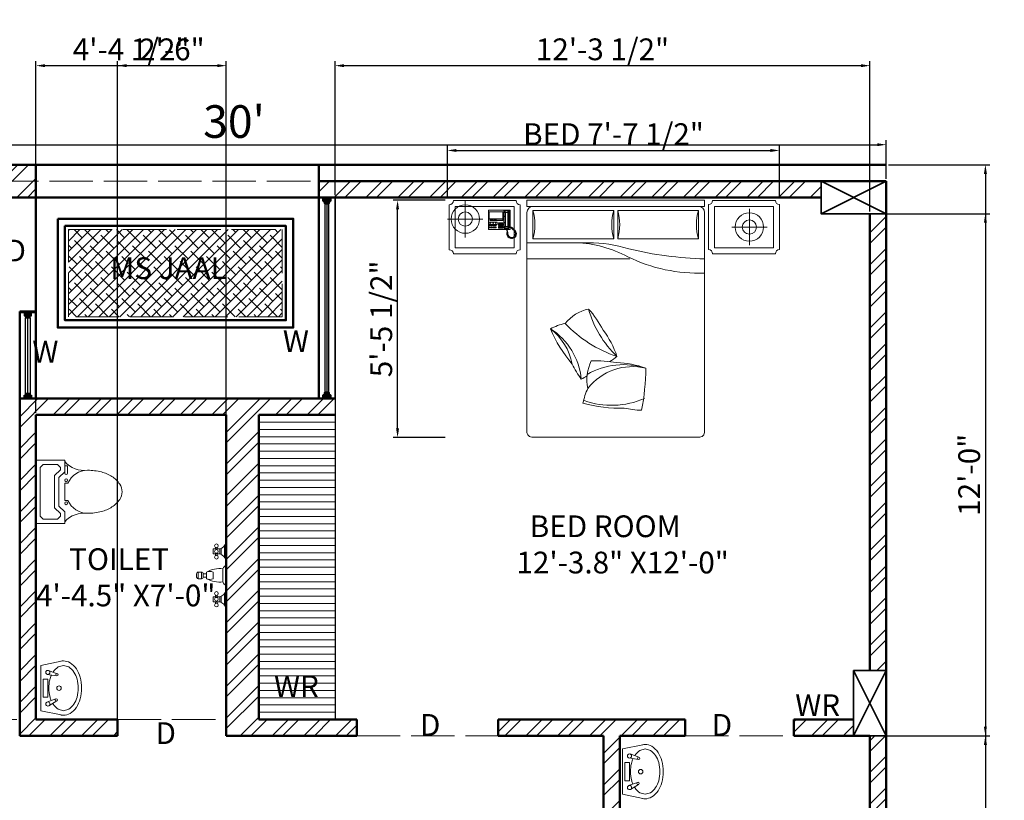
# Model space of a CAD drawing. Units: millimetres. Extents: x 4237 to 5109, y 21391 to 22486.
# Tile 17 of 17: x 4833 to 5105, y 22265 to 22481. Entities that reach past the tile are written whole.
import ezdxf

# ---------------------------------------------------------------- set-up
doc = ezdxf.new("R2010")
doc.units = ezdxf.units.MM
doc.linetypes.add('ACAD_ISO02W100', pattern=[15, 12, -3])
for name, color, linetype, lineweight in [('A-ANNO-DIMS', 2, 'Continuous', 18), ('A-ANNO-TEXT', 7, 'Continuous', 18), ('A-AREA-IDEN', 3, 'Continuous', 18), ('A-FLOR-OVHD', 1, 'ACAD_ISO02W100', 18), ('A-FURN', 8, 'Continuous', 18), ('A-FURN-CASE', 31, 'Continuous', 13), ('A-WALL', 7, 'Continuous', 50), ('A-WALL-PATT', 252, 'Continuous', 13), ('column', 102, 'Continuous', 35), ('windows', 140, 'Continuous', 25)]:
    doc.layers.add(name, color=color, linetype=linetype, lineweight=lineweight)
doc.styles.get("Standard").update_dxf_attribs({"font": 'arial.ttf'})
doc.dimstyles.new('ISO-25', dxfattribs={"dimtxt": 6, "dimasz": 2.5, "dimexe": 1.25, "dimexo": 0.625, "dimtad": 1, "dimdec": 1, "dimlunit": 4, "dimtxsty": 'Standard', "dimcen": 2.5, "dimadec": 0, "dimazin": 0, "dimtfac": 1, "dimtdec": 1, "dimtmove": 0, "dimatfit": 3, "dimfxl": 1, "dimarcsym": 0})

# ---------------------------------------------------------------- blocks, each defined once
blk = doc.blocks.new('A$C07097A50')
for p, q in [((0.0503, 1.9981), (0.5803, 1.9981)), ((0.1513, 1.6872), (0.1513, 1.9968)), ((0.6716, 1.9489), (0.6716, 2.0001)), ((0.6716, 2.0001), (2.1719, 2.0001)), ((2.1719, 1.9489), (2.1719, 2.0001)), ((2.7701, 1.9993), (2.2401, 1.9993)), ((0.0153, 1.9631), (0.0153, 1.5831)), ((0.0653, 1.9481), (0.0653, 1.5981)), ((0.0653, 1.9481), (0.5653, 1.9481)), ((0.3481, 1.9163), (0.3458, 1.914)), ((0.3458, 1.914), (0.3458, 1.7563)), ((0.3481, 1.9163), (0.5287, 1.9163)), ((0.4772, 1.9071), (0.4818, 1.9129)), ((0.4818, 1.9129), (0.5161, 1.9129)), ((0.5161, 1.9129), (0.5218, 1.9071)), ((0.5287, 1.9163), (0.5309, 1.914)), ((0.5309, 1.914), (0.5309, 1.7563)), ((0.5653, 1.9481), (0.5653, 1.5981)), ((0.6153, 1.9631), (0.6153, 1.5831)), ((2.1719, 1.9489), (0.6716, 1.9489)), ((2.2051, 1.9643), (2.2051, 1.5843)), ((2.2551, 1.9493), (2.2551, 1.5993)), ((2.7551, 1.9493), (2.2551, 1.9493)), ((2.5505, 1.6201), (2.5505, 1.9296)), ((2.7551, 1.9493), (2.7551, 1.5993)), ((2.8051, 1.9643), (2.8051, 1.5843)), ((0, 1.8416), (0.3001, 1.8416)), ((0.3526, 1.9037), (0.3526, 1.8431)), ((0.4669, 1.9037), (0.3526, 1.9037)), ((0.3526, 1.8431), (0.4669, 1.8431)), ((0.3572, 1.8409), (0.3572, 1.8294)), ((0.4669, 1.8409), (0.3572, 1.8409)), ((0.3572, 1.8294), (0.4669, 1.8294)), ((0.3664, 1.8409), (0.3664, 1.8294)), ((0.3755, 1.8409), (0.3755, 1.8294)), ((0.3846, 1.8409), (0.3846, 1.8294)), ((0.3938, 1.8409), (0.3938, 1.8294)), ((0.4029, 1.8409), (0.4029, 1.8294)), ((0.4121, 1.8409), (0.4121, 1.8294)), ((0.4669, 1.8431), (0.4669, 1.9037)), ((0.4669, 1.8294), (0.4669, 1.8409)), ((0.4772, 1.7688), (0.4772, 1.9071)), ((0.4818, 1.9094), (0.4807, 1.9049)), ((0.4807, 1.9049), (0.4807, 1.874)), ((0.4807, 1.9049), (0.4909, 1.8946)), ((0.4807, 1.874), (0.4829, 1.8683)), ((0.4864, 1.9117), (0.4818, 1.9094)), ((0.4829, 1.8683), (0.4864, 1.8626)), ((0.4921, 1.8969), (0.4864, 1.9117)), ((0.4864, 1.9117), (0.5138, 1.9117)), ((0.4864, 1.8626), (0.4875, 1.8546)), ((0.4875, 1.8546), (0.4875, 1.8431)), ((0.4875, 1.8214), (0.4875, 1.8431)), ((0.4909, 1.8946), (0.4921, 1.8969)), ((0.4909, 1.8431), (0.4909, 1.8946)), ((0.4909, 1.8431), (0.4909, 1.7814)), ((0.5081, 1.8969), (0.4921, 1.8969)), ((0.5081, 1.8969), (0.5138, 1.9117)), ((0.5092, 1.8946), (0.5081, 1.8969)), ((0.5195, 1.9049), (0.5092, 1.8946)), ((0.5092, 1.8431), (0.5092, 1.8946)), ((0.5092, 1.8431), (0.5092, 1.7814)), ((0.5138, 1.8626), (0.5127, 1.8546)), ((0.5127, 1.8546), (0.5127, 1.8431)), ((0.5127, 1.8214), (0.5127, 1.8431)), ((0.5138, 1.9117), (0.5184, 1.9094)), ((0.5172, 1.8683), (0.5138, 1.8626)), ((0.5195, 1.874), (0.5172, 1.8683)), ((0.5184, 1.9094), (0.5195, 1.9049)), ((0.5195, 1.9049), (0.5195, 1.874)), ((0.5218, 1.9071), (0.5218, 1.77)), ((0.6716, 1.8977), (0.6716, 0.0512)), ((2.1719, 0.0512), (2.1719, 1.8977)), ((0.3458, 1.7563), (0.3481, 1.754)), ((0.5, 1.754), (0.3481, 1.754)), ((0.4201, 1.8168), (0.3526, 1.8168)), ((0.3526, 1.8168), (0.3526, 1.7963)), ((0.3526, 1.7963), (0.4201, 1.7963)), ((0.3652, 1.7906), (0.3538, 1.7906)), ((0.3538, 1.7906), (0.3538, 1.786)), ((0.3538, 1.786), (0.3652, 1.786)), ((0.3538, 1.7666), (0.3538, 1.7734)), ((0.3538, 1.7734), (0.3652, 1.7734)), ((0.3652, 1.7666), (0.3538, 1.7666)), ((0.3675, 1.8146), (0.3641, 1.8146)), ((0.3641, 1.8146), (0.3641, 1.8111)), ((0.3641, 1.8111), (0.3675, 1.8111)), ((0.3641, 1.802), (0.3641, 1.7986)), ((0.3675, 1.802), (0.3641, 1.802)), ((0.3641, 1.7986), (0.3675, 1.7986)), ((0.3652, 1.786), (0.3652, 1.7906)), ((0.3652, 1.7734), (0.3652, 1.7666)), ((0.3675, 1.8111), (0.3675, 1.8146)), ((0.3675, 1.7986), (0.3675, 1.802)), ((0.3812, 1.7906), (0.3698, 1.7906)), ((0.3698, 1.7906), (0.3698, 1.786)), ((0.3698, 1.786), (0.3812, 1.786)), ((0.3698, 1.7666), (0.3698, 1.7734)), ((0.3698, 1.7734), (0.3812, 1.7734)), ((0.3812, 1.7666), (0.3698, 1.7666)), ((0.3812, 1.786), (0.3812, 1.7906)), ((0.3812, 1.7734), (0.3812, 1.7666)), ((0.3846, 1.8146), (0.3846, 1.8111)), ((0.3881, 1.8146), (0.3846, 1.8146)), ((0.3846, 1.8111), (0.3881, 1.8111)), ((0.3846, 1.802), (0.3846, 1.7986)), ((0.3881, 1.802), (0.3846, 1.802)), ((0.3846, 1.7986), (0.3881, 1.7986)), ((0.3972, 1.7906), (0.3858, 1.7906)), ((0.3858, 1.7906), (0.3858, 1.786)), ((0.3858, 1.786), (0.3972, 1.786)), ((0.3858, 1.7666), (0.3858, 1.7734)), ((0.3858, 1.7734), (0.3972, 1.7734)), ((0.3972, 1.7666), (0.3858, 1.7666)), ((0.3881, 1.8111), (0.3881, 1.8146)), ((0.3881, 1.7986), (0.3881, 1.802)), ((0.3972, 1.786), (0.3972, 1.7906)), ((0.3972, 1.7734), (0.3972, 1.7666)), ((0.4018, 1.7906), (0.4018, 1.786)), ((0.4132, 1.7906), (0.4018, 1.7906)), ((0.4018, 1.786), (0.4132, 1.786)), ((0.4018, 1.7734), (0.4132, 1.7734)), ((0.4018, 1.7666), (0.4018, 1.7734)), ((0.4132, 1.7666), (0.4018, 1.7666)), ((0.4052, 1.8146), (0.4052, 1.8111)), ((0.4086, 1.8146), (0.4052, 1.8146)), ((0.4052, 1.8111), (0.4086, 1.8111)), ((0.4052, 1.802), (0.4052, 1.7986)), ((0.4086, 1.802), (0.4052, 1.802)), ((0.4052, 1.7986), (0.4086, 1.7986)), ((0.4086, 1.8111), (0.4086, 1.8146)), ((0.4086, 1.7986), (0.4086, 1.802)), ((0.4132, 1.786), (0.4132, 1.7906)), ((0.4132, 1.7734), (0.4132, 1.7666)), ((0.4201, 1.7963), (0.4201, 1.8168)), ((0.4304, 1.8111), (0.4395, 1.8111)), ((0.4304, 1.8043), (0.4304, 1.8111)), ((0.4395, 1.8043), (0.4304, 1.8043)), ((0.4304, 1.7986), (0.4395, 1.7986)), ((0.4304, 1.7917), (0.4304, 1.7986)), ((0.4395, 1.7917), (0.4304, 1.7917)), ((0.4304, 1.778), (0.4304, 1.7848)), ((0.4304, 1.7848), (0.4395, 1.7848)), ((0.4395, 1.778), (0.4304, 1.778)), ((0.4304, 1.7723), (0.4395, 1.7723)), ((0.4304, 1.7654), (0.4304, 1.7723)), ((0.4395, 1.7654), (0.4304, 1.7654)), ((0.4395, 1.8111), (0.4395, 1.8043)), ((0.4395, 1.7986), (0.4395, 1.7917)), ((0.4395, 1.7848), (0.4395, 1.778)), ((0.4395, 1.7723), (0.4395, 1.7654)), ((0.4441, 1.8043), (0.4441, 1.8111)), ((0.4441, 1.8111), (0.4532, 1.8111)), ((0.4532, 1.8043), (0.4441, 1.8043)), ((0.4441, 1.7986), (0.4532, 1.7986)), ((0.4441, 1.7917), (0.4441, 1.7986)), ((0.4532, 1.7917), (0.4441, 1.7917)), ((0.4441, 1.778), (0.4441, 1.7848)), ((0.4441, 1.7848), (0.4532, 1.7848)), ((0.4532, 1.778), (0.4441, 1.778)), ((0.4441, 1.7723), (0.4532, 1.7723)), ((0.4441, 1.7654), (0.4441, 1.7723)), ((0.4532, 1.7654), (0.4441, 1.7654)), ((0.4532, 1.8111), (0.4532, 1.8043)), ((0.4532, 1.7986), (0.4532, 1.7917)), ((0.4532, 1.7848), (0.4532, 1.778)), ((0.4532, 1.7723), (0.4532, 1.7654)), ((0.4578, 1.8111), (0.4669, 1.8111)), ((0.4578, 1.8043), (0.4578, 1.8111)), ((0.4669, 1.8043), (0.4578, 1.8043)), ((0.4578, 1.7986), (0.4669, 1.7986)), ((0.4578, 1.7917), (0.4578, 1.7986)), ((0.4669, 1.7917), (0.4578, 1.7917)), ((0.4578, 1.7791), (0.4578, 1.786)), ((0.4578, 1.786), (0.4669, 1.786)), ((0.4669, 1.7791), (0.4578, 1.7791)), ((0.4578, 1.7654), (0.4578, 1.7723)), ((0.4578, 1.7723), (0.4669, 1.7723)), ((0.4669, 1.7654), (0.4578, 1.7654)), ((0.4669, 1.8111), (0.4669, 1.8043)), ((0.4669, 1.7986), (0.4669, 1.7917)), ((0.4669, 1.786), (0.4669, 1.7791)), ((0.4669, 1.7723), (0.4669, 1.7654)), ((0.4829, 1.7631), (0.4772, 1.7688)), ((0.4807, 1.802), (0.4829, 1.8077)), ((0.4807, 1.7711), (0.4807, 1.802)), ((0.4807, 1.7711), (0.4909, 1.7814)), ((0.4818, 1.7666), (0.4807, 1.7711)), ((0.4864, 1.7643), (0.4818, 1.7666)), ((0.4829, 1.8077), (0.4864, 1.8134)), ((0.499, 1.7631), (0.4829, 1.7631)), ((0.4864, 1.8134), (0.4875, 1.8214)), ((0.4921, 1.7791), (0.4864, 1.7643)), ((0.4864, 1.7643), (0.499, 1.7643)), ((0.4909, 1.7814), (0.4921, 1.7791)), ((0.5081, 1.7791), (0.4921, 1.7791)), ((0.5024, 1.7677), (0.4989, 1.7677)), ((0.4989, 1.7677), (0.4991, 1.7578)), ((0.4991, 1.7578), (0.5019, 1.7463)), ((0.5019, 1.7463), (0.5047, 1.7354)), ((0.503, 1.7585), (0.5024, 1.7677)), ((0.5026, 1.7643), (0.5138, 1.7643)), ((0.5161, 1.7631), (0.5027, 1.7631)), ((0.5047, 1.7511), (0.503, 1.7585)), ((0.5287, 1.754), (0.504, 1.754)), ((0.5074, 1.7403), (0.5047, 1.7511)), ((0.5092, 1.7814), (0.5081, 1.7791)), ((0.5081, 1.7791), (0.5138, 1.7643)), ((0.5195, 1.7711), (0.5092, 1.7814)), ((0.5138, 1.8134), (0.5127, 1.8214)), ((0.5172, 1.8077), (0.5138, 1.8134)), ((0.5138, 1.7643), (0.5184, 1.7666)), ((0.5218, 1.77), (0.5161, 1.7631)), ((0.5195, 1.802), (0.5172, 1.8077)), ((0.5184, 1.7666), (0.5195, 1.7711)), ((0.5195, 1.7711), (0.5195, 1.802)), ((0.5309, 1.7563), (0.5287, 1.754)), ((0.5378, 1.7743), (0.5309, 1.7768)), ((0.5309, 1.7723), (0.536, 1.7709)), ((0.536, 1.7709), (0.5406, 1.7672)), ((0.541, 1.7711), (0.5378, 1.7743)), ((0.5406, 1.7672), (0.5418, 1.7656)), ((0.5434, 1.7689), (0.541, 1.7711)), ((0.5442, 1.7658), (0.5418, 1.7634)), ((0.5418, 1.7656), (0.5442, 1.7658)), ((0.5418, 1.7634), (0.5511, 1.7552)), ((0.5477, 1.7705), (0.5434, 1.7689)), ((0.5497, 1.7685), (0.5477, 1.7705)), ((0.5481, 1.765), (0.5497, 1.7685)), ((0.5509, 1.7672), (0.5481, 1.765)), ((0.5539, 1.764), (0.5509, 1.7672)), ((0.5511, 1.7552), (0.5662, 1.7423)), ((0.5515, 1.7574), (0.5539, 1.764)), ((0.5577, 1.7606), (0.5515, 1.7574)), ((0.563, 1.7556), (0.5577, 1.7606)), ((0.5618, 1.7483), (0.563, 1.7556)), ((0.567, 1.7515), (0.5618, 1.7483)), ((0.5714, 1.7469), (0.567, 1.7515)), ((0.5696, 1.7419), (0.5714, 1.7469)), ((2.7018, 1.7745), (2.4017, 1.7745)), ((0.5026, 1.7254), (0.5021, 1.7199)), ((0.5021, 1.7199), (0.5088, 1.7187)), ((0.5088, 1.7187), (0.5023, 1.7148)), ((0.5023, 1.7148), (0.5028, 1.7085)), ((0.5051, 1.728), (0.5026, 1.7254)), ((0.5028, 1.7085), (0.5102, 1.7078)), ((0.5102, 1.7078), (0.5037, 1.7028)), ((0.5037, 1.7028), (0.5067, 1.6974)), ((0.5047, 1.7354), (0.5044, 1.7294)), ((0.5044, 1.7294), (0.5051, 1.728)), ((0.5067, 1.6974), (0.5137, 1.6988)), ((0.5081, 1.7347), (0.5074, 1.7403)), ((0.5079, 1.7287), (0.5081, 1.7347)), ((0.5121, 1.7257), (0.5079, 1.7287)), ((0.5137, 1.6988), (0.5104, 1.6923)), ((0.5104, 1.6923), (0.5139, 1.6882)), ((0.5111, 1.7203), (0.5121, 1.7257)), ((0.5123, 1.7058), (0.5111, 1.7203)), ((0.5211, 1.6947), (0.5123, 1.7058)), ((0.5139, 1.6882), (0.5192, 1.6921)), ((0.5192, 1.6921), (0.5183, 1.6859)), ((0.5183, 1.6859), (0.5227, 1.6831)), ((0.5333, 1.6882), (0.5211, 1.6947)), ((0.5227, 1.6831), (0.5282, 1.6877)), ((0.5282, 1.6877), (0.5276, 1.6801)), ((0.5276, 1.6801), (0.5324, 1.6787)), ((0.5324, 1.6787), (0.5354, 1.6849)), ((0.5472, 1.687), (0.5333, 1.6882)), ((0.5354, 1.6849), (0.5382, 1.6787)), ((0.5382, 1.6787), (0.5421, 1.6782)), ((0.5421, 1.6782), (0.5437, 1.6849)), ((0.5437, 1.6849), (0.5463, 1.6775)), ((0.5463, 1.6775), (0.5507, 1.6787)), ((0.5606, 1.6928), (0.5472, 1.687)), ((0.5507, 1.6787), (0.5509, 1.6849)), ((0.5509, 1.6849), (0.5562, 1.6803)), ((0.5562, 1.6803), (0.5599, 1.6822)), ((0.5592, 1.6891), (0.5641, 1.6831)), ((0.5599, 1.6822), (0.5592, 1.6891)), ((0.5708, 1.7028), (0.5606, 1.6928)), ((0.5641, 1.6831), (0.5678, 1.6863)), ((0.565, 1.6926), (0.5715, 1.6898)), ((0.5678, 1.6863), (0.565, 1.6926)), ((0.5664, 1.7419), (0.574, 1.7201)), ((0.5766, 1.7426), (0.5697, 1.7419)), ((0.574, 1.7201), (0.5708, 1.7028)), ((0.5745, 1.6926), (0.5713, 1.6988)), ((0.5713, 1.6988), (0.578, 1.6967)), ((0.5715, 1.6898), (0.5745, 1.6926)), ((0.572, 1.7331), (0.5787, 1.7356)), ((0.5794, 1.7333), (0.572, 1.7331)), ((0.5743, 1.7076), (0.5814, 1.7074)), ((0.5798, 1.7014), (0.5743, 1.7076)), ((0.5761, 1.7234), (0.581, 1.728)), ((0.5824, 1.7234), (0.5761, 1.7234)), ((0.5764, 1.7155), (0.5835, 1.7176)), ((0.5824, 1.712), (0.5764, 1.7155)), ((0.5787, 1.7356), (0.5766, 1.7426)), ((0.578, 1.6967), (0.5798, 1.7014)), ((0.581, 1.728), (0.5794, 1.7333)), ((0.5814, 1.7074), (0.5824, 1.712)), ((0.5835, 1.7176), (0.5824, 1.7234)), ((0.0653, 1.5981), (0.5653, 1.5981)), ((2.7551, 1.5993), (2.2551, 1.5993)), ((0.0503, 1.5481), (0.5803, 1.5481)), ((2.7701, 1.5493), (2.2401, 1.5493)), ((0.7228, 0.0001), (2.1207, 0.0001))]:
    blk.add_line(p, q)
at = {"linetype": 'ByBlock'}
for p, q in [((0.7228, 1.6759), (0.7228, 1.9148)), ((0.7228, 1.9148), (1.4047, 1.9148)), ((1.4047, 1.9148), (1.4047, 1.6759)), ((1.4388, 1.6759), (1.4388, 1.9148)), ((1.4388, 1.9148), (2.1207, 1.9148)), ((2.1207, 1.9148), (2.1207, 1.6759)), ((1.4047, 1.6759), (0.7228, 1.6759)), ((2.1207, 1.6759), (1.4388, 1.6759)), ((1.1914, 1.6418), (0.6716, 1.6418)), ((1.5412, 1.5053), (0.6716, 1.5053))]:
    blk.add_line(p, q, dxfattribs=at)
for centre in [(0.1513, 1.8416), (2.5505, 1.7745)]:
    blk.add_circle(centre, 0.12, dxfattribs=at)
for centre in [(0.1513, 1.8416), (2.5505, 1.7745)]:
    blk.add_circle(centre, 0.06)
for centre, radius, start, end in [((0.0153, 1.9981), 0.035, 270, 0), ((0.6153, 1.9981), 0.035, 180, 270), ((2.2051, 1.9993), 0.035, 270, 0), ((2.8051, 1.9993), 0.035, 180, 270), ((0.7228, 1.8977), 0.0512, 90, 180), ((2.1207, 1.8977), 0.0512, 0, 90), ((0.0153, 1.5481), 0.035, 0, 90), ((0.6153, 1.5481), 0.035, 90, 180), ((2.2051, 1.5493), 0.035, 0, 90), ((2.8051, 1.5493), 0.035, 90, 180), ((1.2698, 0.7333), 0.3575, 102.47819, 140.46254), ((0.4476, 0.4335), 0.9879, 28.49711, 41.05657), ((2.0313, 1.3124), 0.8697, 195.33601, 226.41927), ((1.1192, 0.4274), 0.548, 103.20343, 117.03623), ((1.9422, 1.372), 1.1652, 203.06416, 220.32086), ((0.5744, 0.5274), 0.4879, 10.69865, 52.68638), ((0.5678, 0.4375), 0.5655, 5.33912, 57.68949), ((1.7756, 1.7059), 1.0798, 223.63057, 251.4288), ((0.6844, 0.4345), 0.7874, 18.35266, 36.68512), ((0.1017, 2.4319), 2.1977, 305.29657, 307.24182), ((1.7177, 0.9312), 0.734, 205.25901, 216.93514), ((1.5362, 0.487), 0.3575, 154.0418, 192.02615), ((1.4868, 0.0041), 0.6085, 71.81005, 120.13512), ((1.5627, 0.1186), 0.4774, 76.18494, 142.00166), ((1.2599, -0.3434), 0.9879, 80.06073, 92.62018), ((1.4063, -0.1573), 0.7874, 69.91627, 88.24873), ((-0.5205, 0.628), 2.1977, 349.48843, 358.80544), ((0.1017, 2.4319), 2.1977, 297.92482, 299.3793), ((1.6822, 0.1789), 0.548, 154.76704, 168.59984), ((1.4539, 1.4107), 1.1652, 254.62778, 271.88448), ((1.3874, 0.9578), 0.6885, 250.29361, 293.6414), ((1.6595, 0.9609), 0.734, 256.82263, 268.49876), ((0.717, 0.0455), 0.0458, 172.75992, 277.24008), ((2.1265, 0.0455), 0.0458, 262.75992, 7.24008)]:
    blk.add_arc(centre, radius, start, end)
for centre, radius, start, end in [((0.3133, 1.7953), 0.4265, 343.73979, 16.26021), ((1.8141, 1.7953), 0.4265, 163.73979, 196.26021), ((1.0294, 1.7953), 0.4265, 343.73979, 16.26021), ((2.5302, 1.7953), 0.4265, 163.73979, 196.26021), ((1.053, 0.6571), 0.9853, 61.43285, 88.12613), ((1.2053, 0.5713), 1.0706, 72.19663, 90.74184), ((2.2595, 4.5996), 3.0955, 256.42012, 268.37887), ((2.1283, 2.7745), 1.3903, 244.24266, 271.79845)]:
    blk.add_arc(centre, radius, start, end, dxfattribs=at)
blk = doc.blocks.new('A$C5EF6120A')
at = {"linetype": 'ByBlock'}
for p, q in [((0, 0.762), (0, 0.508)), ((0, 0.762), (0.5588, 0.762)), ((0.0381, 0.6985), (0.0635, 0.7239)), ((0.0381, 0.6985), (0.0381, 0.5715)), ((0.0635, 0.7239), (0.4953, 0.7239)), ((0.4953, 0.7239), (0.5207, 0.6985)), ((0.5207, 0.6985), (0.5207, 0.5715)), ((0.5588, 0.762), (0.5588, 0.508)), ((0.0635, 0.5461), (0.0381, 0.5715)), ((0.0635, 0.5461), (0.0858, 0.5461)), ((0.1366, 0.5969), (0.0858, 0.5461)), ((0.1524, 0.5588), (0.1016, 0.508)), ((0.1366, 0.5969), (0.4222, 0.5969)), ((0.1524, 0.5588), (0.4064, 0.5588)), ((0.4064, 0.5588), (0.4572, 0.508)), ((0.4222, 0.5969), (0.473, 0.5461)), ((0.4953, 0.5461), (0.473, 0.5461)), ((0.5207, 0.5715), (0.4953, 0.5461)), ((0, 0.508), (0.1016, 0.508)), ((0.0508, 0.508), (0.0508, 0.4826)), ((0.0508, 0.4826), (0.1143, 0.4826)), ((0.1143, 0.508), (0.1016, 0.508)), ((0.2032, 0.508), (0.2032, 0.4794)), ((0.3556, 0.508), (0.2032, 0.508)), ((0.3556, 0.508), (0.3556, 0.4794)), ((0.5588, 0.508), (0.4572, 0.508))]:
    blk.add_line(p, q, dxfattribs=at)
blk.add_lwpolyline([(0.0889, 0.3048, 0.063415), (0.1044, 0.183, 0.076468), (0.1447, 0.0893, 0.107136), (0.2118, 0.0204, 0.147373), (0.2794, 0, 0.147373), (0.347, 0.0204, 0.107136), (0.4141, 0.0893, 0.076468), (0.4544, 0.183, 0.063415), (0.4699, 0.3048, 0.063415)], format="xyb", dxfattribs=at)
for centre in [(0.1778, 0.4953), (0.381, 0.4953)]:
    blk.add_circle(centre, 0.0127, dxfattribs=at)
for centre, radius, start, end in [((-0.1375, 0.3358), 0.2285, 352.20108, 48.91101), ((0.2794, 0.3048), 0.1905, 113.57818, 180), ((0.1143, 0.4953), 0.0127, 270, 90), ((0.2794, 0.3048), 0.1905, 0, 66.42182), ((0.6963, 0.3358), 0.2285, 131.08899, 187.79892)]:
    blk.add_arc(centre, radius, start, end, dxfattribs=at)
blk = doc.blocks.new('A$C60F95712')
for p, q in [((0.05, 0.45), (0.003, 0.228)), ((0.55, 0.45), (0.05, 0.45)), ((0.597, 0.228), (0.55, 0.45)), ((0.103, 0.364), (0.159, 0.273)), ((0.145, 0.383), (0.181, 0.284)), ((0.4, 0.425), (0.2, 0.425)), ((0.2, 0.425), (0.2, 0.375)), ((0.2, 0.375), (0.4, 0.375)), ((0.4, 0.375), (0.4, 0.425)), ((0.451, 0.38), (0.435, 0.275)), ((0.495, 0.368), (0.459, 0.269))]:
    blk.add_line(p, q)
for points in [[(0.444, 0.333, 0.046779), (0.391, 0.352, 0.080145), (0.3, 0.362, 0.065516), (0.2, 0.349, 0.037125), (0.162, 0.335, 0.107176)], [(0.131, 0.319, 0.008163), (0.123, 0.314, 0.107176), (0.067, 0.258), (0.05, 0.2), (0.067, 0.142, 0.107176), (0.123, 0.086, 0.078233), (0.2, 0.051, 0.065516), (0.3, 0.038, 0.065516), (0.4, 0.051, 0.078233), (0.477, 0.086, 0.107176), (0.533, 0.142), (0.55, 0.2)], [(0.55, 0.2), (0.533, 0.258, 0.107176), (0.477, 0.314, 0.000976), (0.476, 0.315, 0.080145)]]:
    blk.add_lwpolyline(points, format="xyb")
for centre, radius in [((0.124, 0.373), 0.0228), ((0.473, 0.374), 0.0228), ((0.17, 0.279), 0.0126), ((0.3, 0.25), 0.025), ((0.447, 0.273), 0.0126)]:
    blk.add_circle(centre, radius)
for centre, radius, start, end in [((0.136, 0.2), 0.136, 168.024, 180), ((0.464, 0.2), 0.136, 0, 11.976), ((0.136, 0.2), 0.136, 180, 211.8535), ((0.215, 0.249), 0.229, 211.8535, 236.3099), ((0.385, 0.249), 0.229, 303.6901, 328.1465), ((0.464, 0.2), 0.136, 328.1465, 0), ((0.266, 0.326), 0.322, 236.3099, 254.5629), ((0.3, 0.448), 0.448, 254.5629, 270), ((0.3, 0.448), 0.448, 270, 285.4371), ((0.334, 0.326), 0.322, 285.4371, 303.6901)]:
    blk.add_arc(centre, radius, start, end)
blk = doc.blocks.new('Faucet - Bathroom front')
for p, q in [((-0.5, 4.25), (0.5, 4.25)), ((0.5, 3.75), (-0.5, 3.75)), ((-0.5, 3), (0.5, 3)), ((-0.25, 3), (-0.25, 3.5)), ((0.25, 3.5), (0.25, 3)), ((-4, 1.625), (-4.25, 1.625)), ((-3.25, 1.625), (-3, 1.625)), ((0.5, 2), (-0.5, 2)), ((3.25, 1.625), (3, 1.625)), ((4, 1.625), (4.25, 1.625)), ((-5, 0), (-2.25, 0)), ((-4.5087, 0.25), (-2.7408, 0.25)), ((-4, 1.375), (-4.25, 1.375)), ((-3.1442, 0.75), (-4.0979, 0.75)), ((-3.25, 1.375), (-3, 1.375)), ((-1.5, 0), (1.5, 0)), ((-1, 0.5), (1, 0.5)), ((2.25, 0), (5, 0)), ((2.7413, 0.25), (4.5092, 0.25)), ((3.25, 1.375), (3, 1.375)), ((4.1058, 0.75), (3.1521, 0.75)), ((4, 1.375), (4.25, 1.375))]:
    blk.add_line(p, q)
for points in [[(-0.25, 4.5), (0.25, 4.5)], [(-0.5, 3.75), (-0.5, 4.25)], [(0.25, 3.5), (-0.25, 3.5)], [(0.5, 4.25), (0.5, 3.75)]]:
    blk.add_lwpolyline(points)
for points in [[(-4, 1), (-4, 2), (-3.25, 2), (-3.25, 1)], [(3.25, 1), (3.25, 2), (4, 2), (4, 1)]]:
    blk.add_lwpolyline(points, close=True)
for centre in [(-4.5, 1.5), (-3.625, 1.5), (-2.75, 1.5), (2.75, 1.5), (3.625, 1.5), (4.5, 1.5)]:
    blk.add_circle(centre, 0.2795)
for centre, radius, start, end in [((-0.2575, 4.2575), 0.2426, 88.22243, 181.7776), ((0.2575, 4.2575), 0.2426, 358.2224, 91.77757), ((3, 1), 4.0311, 150.2551, 187.125), ((0.6413, 2.5), 1.246, 156.3417, 203.6583), ((-0.2575, 3.7425), 0.2426, 178.2224, 271.7776), ((0.2575, 3.7425), 0.2426, 268.2224, 1.777565), ((-3, 1), 4.0311, 352.875, 29.74488), ((-0.6413, 2.5), 1.246, 336.3417, 23.65835), ((-5.375, 1.375), 1.4252, 285.2551, 344.7449), ((-1.875, 1.375), 1.4252, 195.2551, 254.7449), ((-0.7962, -0.2038), 0.7327, 106.1502, 163.8498), ((0.7962, -0.2038), 0.7327, 16.1502, 73.84979), ((1.875, 1.375), 1.4252, 285.2551, 344.7449), ((5.375, 1.375), 1.4252, 195.2551, 254.7449)]:
    blk.add_arc(centre, radius, start, end)
blk = doc.blocks.new('*D59')
at = {"layer": 'A-ANNO-DIMS', "color": 0, "lineweight": -2, "transparency": 16777216}
for p, q in [((4712.61, 22441.33), (4712.61, 22447.5)), ((4715.11, 22446.25), (5070.01, 22446.25)), ((5072.51, 22436.83), (5072.51, 22447.5))]:
    blk.add_line(p, q, dxfattribs=at)
at = {"layer": 'A-ANNO-DIMS', "color": 0, "transparency": 16777216}
for points in [[(4715.11, 22446.66), (4715.11, 22445.83), (4712.61, 22446.25)], [(5070.01, 22446.66), (5070.01, 22445.83), (5072.51, 22446.25)]]:
    blk.add_solid(points, dxfattribs=at)
at = {"layer": 'Defpoints', "color": 0, "transparency": 16777216}
for p in [(5072.51, 22446.25), (4712.61, 22440.7), (5072.51, 22436.2)]:
    blk.add_point(p, dxfattribs=at)
at = {"layer": 'A-ANNO-DIMS', "color": 0, "transparency": 16777216, "insert": (4892.56, 22451.47), "char_height": 9, "attachment_point": 5}
blk.add_mtext("30'", dxfattribs=at)
blk = doc.blocks.new('COLUMN-X')
blk.add_line((18, 9), (0, 0))
blk.add_lwpolyline([(18, 9), (0, 9), (0, 0), (18, 0)], close=True)
blk = doc.blocks.new('*D70')
at = {"layer": 'A-ANNO-DIMS', "color": 0, "lineweight": -2, "transparency": 16777216}
for p, q in [((4951.42, 22431.53), (4951.42, 22445.91)), ((5043.07, 22431.53), (5043.07, 22445.91)), ((4953.92, 22444.66), (5040.57, 22444.66))]:
    blk.add_line(p, q, dxfattribs=at)
at = {"layer": 'A-ANNO-DIMS', "color": 0, "transparency": 16777216}
for points in [[(4953.92, 22445.07), (4953.92, 22444.24), (4951.42, 22444.66)], [(5040.57, 22445.07), (5040.57, 22444.24), (5043.07, 22444.66)]]:
    blk.add_solid(points, dxfattribs=at)
at = {"layer": 'Defpoints', "color": 0, "transparency": 16777216}
for p in [(5043.07, 22444.66), (4951.42, 22430.91), (5043.07, 22430.91)]:
    blk.add_point(p, dxfattribs=at)
at = {"layer": 'A-ANNO-DIMS', "color": 0, "transparency": 16777216, "insert": (4997.25, 22448.38), "char_height": 6, "attachment_point": 5}
blk.add_mtext('BED 7\'-7 1/2"', dxfattribs=at)
blk = doc.blocks.new('*D71')
at = {"layer": 'A-ANNO-DIMS', "color": 0, "lineweight": -2, "transparency": 16777216}
for p, q in [((4950.8, 22430.91), (4936.43, 22430.91)), ((4937.68, 22368.01), (4937.68, 22428.41)), ((4950.8, 22365.51), (4936.43, 22365.51))]:
    blk.add_line(p, q, dxfattribs=at)
at = {"layer": 'A-ANNO-DIMS', "color": 0, "transparency": 16777216}
for points in [[(4937.26, 22428.41), (4938.09, 22428.41), (4937.68, 22430.91)], [(4937.26, 22368.01), (4938.09, 22368.01), (4937.68, 22365.51)]]:
    blk.add_solid(points, dxfattribs=at)
at = {"layer": 'Defpoints', "color": 0, "transparency": 16777216}
for p in [(4937.68, 22430.91), (4951.42, 22430.91), (4951.42, 22365.51)]:
    blk.add_point(p, dxfattribs=at)
at = {"layer": 'A-ANNO-DIMS', "color": 0, "transparency": 16777216, "insert": (4933.95, 22398.21), "char_height": 6, "attachment_point": 5, "rotation": 90}
blk.add_mtext('5\'-5 1/2"', dxfattribs=at)
blk = doc.blocks.new('*D114')
at = {"layer": 'A-ANNO-DIMS', "color": 0, "lineweight": -2, "transparency": 16777216}
for p, q in [((4837.91, 22372.33), (4837.91, 22469.3)), ((4840.41, 22468.05), (4887.91, 22468.05)), ((4890.41, 22372.33), (4890.41, 22469.3))]:
    blk.add_line(p, q, dxfattribs=at)
at = {"layer": 'A-ANNO-DIMS', "color": 0, "transparency": 16777216}
for points in [[(4840.41, 22468.47), (4840.41, 22467.63), (4837.91, 22468.05)], [(4887.91, 22468.47), (4887.91, 22467.63), (4890.41, 22468.05)]]:
    blk.add_solid(points, dxfattribs=at)
at = {"layer": 'Defpoints', "color": 0, "transparency": 16777216}
for p in [(4890.41, 22468.05), (4837.91, 22371.7), (4890.41, 22371.7)]:
    blk.add_point(p, dxfattribs=at)
at = {"layer": 'A-ANNO-DIMS', "color": 0, "transparency": 16777216, "insert": (4864.16, 22471.78), "char_height": 6, "attachment_point": 5}
blk.add_mtext('4\'-4 1/2"', dxfattribs=at)
blk = doc.blocks.new('*D115')
at = {"layer": 'A-ANNO-DIMS', "color": 0, "lineweight": -2, "transparency": 16777216}
for p, q in [((4920.41, 22432.33), (4920.41, 22469.3)), ((4922.91, 22468.05), (5065.51, 22468.05)), ((5068.01, 22427.83), (5068.01, 22469.3))]:
    blk.add_line(p, q, dxfattribs=at)
at = {"layer": 'A-ANNO-DIMS', "color": 0, "transparency": 16777216}
for points in [[(4922.91, 22468.47), (4922.91, 22467.63), (4920.41, 22468.05)], [(5065.51, 22468.47), (5065.51, 22467.63), (5068.01, 22468.05)]]:
    blk.add_solid(points, dxfattribs=at)
at = {"layer": 'Defpoints', "color": 0, "transparency": 16777216}
for p in [(5068.01, 22468.05), (4920.41, 22431.7), (5068.01, 22427.2)]:
    blk.add_point(p, dxfattribs=at)
at = {"layer": 'A-ANNO-DIMS', "color": 0, "transparency": 16777216, "insert": (4994.21, 22471.78), "char_height": 6, "attachment_point": 5}
blk.add_mtext('12\'-3 1/2"', dxfattribs=at)
blk = doc.blocks.new('*D116')
at = {"layer": 'A-ANNO-DIMS', "color": 0, "lineweight": -2, "transparency": 16777216}
for p, q in [((5073.14, 22440.7), (5101.11, 22440.7)), ((5099.86, 22438.2), (5099.86, 21979.7)), ((5073.14, 21977.2), (5101.11, 21977.2))]:
    blk.add_line(p, q, dxfattribs=at)
at = {"layer": 'A-ANNO-DIMS', "color": 0, "transparency": 16777216}
for points in [[(5099.45, 22438.2), (5100.28, 22438.2), (5099.86, 22440.7)], [(5099.45, 21979.7), (5100.28, 21979.7), (5099.86, 21977.2)]]:
    blk.add_solid(points, dxfattribs=at)
at = {"layer": 'Defpoints', "color": 0, "transparency": 16777216}
for p in [(5072.51, 22440.7), (5072.51, 21977.2), (5099.86, 21977.2)]:
    blk.add_point(p, dxfattribs=at)
at = {"layer": 'A-ANNO-DIMS', "color": 0, "transparency": 16777216, "insert": (5096.13, 22208.95), "char_height": 6, "attachment_point": 5, "rotation": 90}
blk.add_mtext('38\'-7 1/2"', dxfattribs=at)
blk = doc.blocks.new('*D117')
at = {"layer": 'A-ANNO-DIMS', "color": 0, "lineweight": -2, "transparency": 16777216}
for p, q in [((5068.64, 22427.2), (5101.11, 22427.2)), ((5099.86, 22424.7), (5099.86, 22285.7)), ((5068.64, 22283.2), (5101.11, 22283.2))]:
    blk.add_line(p, q, dxfattribs=at)
at = {"layer": 'A-ANNO-DIMS', "color": 0, "transparency": 16777216}
for points in [[(5099.45, 22424.7), (5100.28, 22424.7), (5099.86, 22427.2)], [(5099.45, 22285.7), (5100.28, 22285.7), (5099.86, 22283.2)]]:
    blk.add_solid(points, dxfattribs=at)
at = {"layer": 'Defpoints', "color": 0, "transparency": 16777216}
for p in [(5068.01, 22427.2), (5068.01, 22283.2), (5099.86, 22283.2)]:
    blk.add_point(p, dxfattribs=at)
at = {"layer": 'A-ANNO-DIMS', "color": 0, "transparency": 16777216, "insert": (5096.17, 22355.2), "char_height": 6, "attachment_point": 5, "rotation": 90}
blk.add_mtext('12\'-0"', dxfattribs=at)
blk = doc.blocks.new('*D118')
at = {"layer": 'A-ANNO-DIMS', "color": 0, "lineweight": -2, "transparency": 16777216}
for p, q in [((5068.64, 22283.2), (5101.11, 22283.2)), ((5099.86, 22280.7), (5099.86, 22137.2)), ((5064.14, 22134.7), (5101.11, 22134.7))]:
    blk.add_line(p, q, dxfattribs=at)
at = {"layer": 'A-ANNO-DIMS', "color": 0, "transparency": 16777216}
for points in [[(5099.45, 22280.7), (5100.28, 22280.7), (5099.86, 22283.2)], [(5099.45, 22137.2), (5100.28, 22137.2), (5099.86, 22134.7)]]:
    blk.add_solid(points, dxfattribs=at)
at = {"layer": 'Defpoints', "color": 0, "transparency": 16777216}
for p in [(5068.01, 22283.2), (5063.51, 22134.7), (5099.86, 22134.7)]:
    blk.add_point(p, dxfattribs=at)
at = {"layer": 'A-ANNO-DIMS', "color": 0, "transparency": 16777216, "insert": (5096.13, 22208.95), "char_height": 6, "attachment_point": 5, "rotation": 90}
blk.add_mtext('12\'-4 1/2"', dxfattribs=at)
blk = doc.blocks.new('*D121')
at = {"layer": 'A-ANNO-DIMS', "color": 0, "lineweight": -2, "transparency": 16777216}
for p, q in [((4860.41, 22283.83), (4860.41, 22469.3)), ((4862.91, 22468.05), (4887.91, 22468.05)), ((4890.41, 22283.83), (4890.41, 22469.3))]:
    blk.add_line(p, q, dxfattribs=at)
at = {"layer": 'A-ANNO-DIMS', "color": 0, "transparency": 16777216}
for points in [[(4862.91, 22468.47), (4862.91, 22467.63), (4860.41, 22468.05)], [(4887.91, 22468.47), (4887.91, 22467.63), (4890.41, 22468.05)]]:
    blk.add_solid(points, dxfattribs=at)
at = {"layer": 'Defpoints', "color": 0, "transparency": 16777216}
for p in [(4890.41, 22468.05), (4860.41, 22283.2), (4890.41, 22283.2)]:
    blk.add_point(p, dxfattribs=at)
at = {"layer": 'A-ANNO-DIMS', "color": 0, "transparency": 16777216, "insert": (4875.41, 22471.74), "char_height": 6, "attachment_point": 5}
blk.add_mtext('2\'-6"', dxfattribs=at)

msp = doc.modelspace()

# ---------------------------------------------------------------- hatches: boundary and pattern name
at = {"layer": 'A-WALL-PATT'}
h = msp.add_hatch(dxfattribs=at)
h.set_pattern_fill('ANSI32', color=256, scale=0.65)
h.paths.add_polyline_path([(4837.91, 22440.7), (4721.61, 22440.7), (4721.61, 22431.7), (4837.91, 22431.7)])
h = msp.add_hatch(dxfattribs=at)
h.set_pattern_fill('ANSI32', color=256, scale=0.65)
h.paths.add_polyline_path([(5054.51, 22436.2), (4915.91, 22436.2), (4915.91, 22431.7), (5054.51, 22431.7)])
h = msp.add_hatch(color=256, dxfattribs=at)
h.dxf.hatch_style = 1
h.paths.add_polyline_path([(4919.16, 22431.7), (4917.16, 22431.7), (4917.16, 22430.7), (4917.62, 22430.7), (4917.62, 22430), (4918.7, 22430), (4918.7, 22430.7), (4919.16, 22430.7)])
h = msp.add_hatch(dxfattribs=at)
h.set_pattern_fill('ANSI32', color=256, scale=0.65)
h.paths.add_polyline_path([(5072.51, 22427.2), (5068.01, 22427.2), (5068.01, 22301.2), (5072.51, 22301.2)])
h = msp.add_hatch(dxfattribs=at)
h.set_pattern_fill('ANSI38', color=256, scale=0.65)
h.paths.add_polyline_path([(4905.87, 22422.84), (4846.89, 22422.84), (4846.89, 22398.81), (4905.87, 22398.81)])
h.paths.add_polyline_path([(4855.07, 22405.81), (4895.34, 22405.81), (4895.34, 22418.18), (4855.07, 22418.18)], flags=24)
h = msp.add_hatch(color=256, dxfattribs=at)
h.dxf.hatch_style = 1
h.paths.add_polyline_path([(4836.66, 22400), (4834.66, 22400), (4834.66, 22399), (4835.05, 22399), (4835.05, 22398.49), (4836.27, 22398.49), (4836.27, 22399), (4836.66, 22399)])
h = msp.add_hatch(color=256, dxfattribs=at)
h.dxf.hatch_style = 1
h.paths.add_polyline_path([(4836.66, 22377.2), (4836.27, 22377.2), (4836.27, 22377.71), (4835.05, 22377.71), (4835.05, 22377.2), (4834.66, 22377.2), (4834.66, 22376.2), (4836.66, 22376.2)])
h = msp.add_hatch(color=256, dxfattribs=at)
h.dxf.hatch_style = 1
h.paths.add_polyline_path([(4919.16, 22377.2), (4918.7, 22377.2), (4918.7, 22377.9), (4917.62, 22377.9), (4917.62, 22377.2), (4917.16, 22377.2), (4917.16, 22376.2), (4919.16, 22376.2)], flags=17)
h = msp.add_hatch(dxfattribs=at)
h.set_pattern_fill('ANSI32', color=256, scale=0.65)
h.paths.add_polyline_path([(4926.41, 22287.7), (4899.41, 22287.7), (4899.41, 22371.7), (4920.41, 22371.7), (4920.41, 22376.2), (4915.91, 22376.2), (4833.41, 22376.2), (4833.41, 22283.2), (4860.41, 22283.2), (4860.41, 22287.7), (4837.91, 22287.7), (4837.91, 22371.7), (4890.41, 22371.7), (4890.41, 22283.2), (4926.41, 22283.2)])
h = msp.add_hatch(dxfattribs=at)
h.set_pattern_fill('ANSI32', color=256, scale=0.65)
h.paths.add_polyline_path([(5045.51, 22223.2), (5051.51, 22223.2), (5051.51, 22227.7), (5041.01, 22227.7), (5041.01, 22211.2), (4999.01, 22211.2), (4999.01, 22283.2), (5017.01, 22283.2), (5017.01, 22287.7), (4965.41, 22287.7), (4965.41, 22283.2), (4994.51, 22283.2), (4994.51, 22134.7), (4938.41, 22134.7), (4938.41, 22130.2), (5011.33, 22130.2), (5011.33, 22134.7), (4999.01, 22134.7), (4999.01, 22206.7), (5041.01, 22206.7), (5041.01, 22190.2), (5051.51, 22190.2), (5051.51, 22194.7), (5045.51, 22194.7)])
h = msp.add_hatch(dxfattribs=at)
h.set_pattern_fill('ANSI32', color=256, scale=0.65)
h.paths.add_polyline_path([(5063.51, 22287.7), (5047.01, 22287.7), (5047.01, 22283.2), (5063.51, 22283.2)], flags=17)
h = msp.add_hatch(dxfattribs=at)
h.set_pattern_fill('ANSI32', color=256, scale=0.65)
h.paths.add_polyline_path([(5072.51, 22283.2), (5068.01, 22283.2), (5068.01, 22144), (5072.51, 22144)])

# ---------------------------------------------------------------- linework, layer by layer
at = {"layer": 'A-FLOR-OVHD'}
for p, q in [((4721.61, 22436.2), (4915.91, 22436.2)), ((4790.61, 22287.7), (4833.41, 22287.7)), ((4860.41, 22287.7), (4890.41, 22287.7)), ((4926.41, 22283.2), (4965.41, 22283.2)), ((5017.01, 22283.2), (5047.01, 22283.2))]:
    msp.add_line(p, q, dxfattribs=at)
msp.add_lwpolyline([(4846.89, 22422.84), (4905.87, 22422.84), (4905.87, 22398.81), (4846.89, 22398.81)], close=True, dxfattribs=at)
at = {"layer": 'A-FURN-CASE'}
for p, q in [((4899.41, 22369.7), (4920.41, 22369.7)), ((4899.41, 22367.7), (4920.41, 22367.7)), ((4899.41, 22365.7), (4920.41, 22365.7)), ((4899.41, 22363.7), (4920.41, 22363.7)), ((4899.41, 22361.7), (4920.41, 22361.7)), ((4899.41, 22359.7), (4920.41, 22359.7)), ((4899.41, 22357.7), (4920.41, 22357.7)), ((4899.41, 22355.7), (4920.41, 22355.7)), ((4899.41, 22353.7), (4920.41, 22353.7)), ((4899.41, 22351.7), (4920.41, 22351.7)), ((4899.41, 22349.7), (4920.41, 22349.7)), ((4899.41, 22347.7), (4920.41, 22347.7)), ((4899.41, 22345.7), (4920.41, 22345.7)), ((4899.41, 22343.7), (4920.41, 22343.7)), ((4899.41, 22341.7), (4920.41, 22341.7)), ((4899.41, 22339.7), (4920.41, 22339.7)), ((4899.41, 22337.7), (4920.41, 22337.7)), ((4899.41, 22335.7), (4920.41, 22335.7)), ((4899.41, 22333.7), (4920.41, 22333.7)), ((4899.41, 22331.7), (4920.41, 22331.7)), ((4899.41, 22329.7), (4920.41, 22329.7)), ((4899.41, 22327.7), (4920.41, 22327.7)), ((4899.41, 22325.7), (4920.41, 22325.7)), ((4899.41, 22323.7), (4920.41, 22323.7)), ((4899.41, 22321.7), (4920.41, 22321.7)), ((4899.41, 22319.7), (4920.41, 22319.7)), ((4899.41, 22317.7), (4920.41, 22317.7)), ((4899.41, 22315.7), (4920.41, 22315.7)), ((4899.41, 22313.7), (4920.41, 22313.7)), ((4899.41, 22311.7), (4920.41, 22311.7)), ((4899.41, 22309.7), (4920.41, 22309.7)), ((4899.41, 22307.7), (4920.41, 22307.7)), ((4899.41, 22305.7), (4920.41, 22305.7)), ((4899.41, 22303.7), (4920.41, 22303.7)), ((4899.41, 22301.7), (4920.41, 22301.7)), ((4899.41, 22299.7), (4920.41, 22299.7)), ((4899.41, 22297.7), (4920.41, 22297.7)), ((4899.41, 22295.7), (4920.41, 22295.7)), ((4899.41, 22293.7), (4920.41, 22293.7)), ((4899.41, 22291.7), (4920.41, 22291.7)), ((4899.41, 22289.7), (4920.41, 22289.7))]:
    msp.add_line(p, q, dxfattribs=at)
at = {"layer": 'A-WALL'}
for p, q in [((4712.61, 22440.7), (4837.91, 22440.7)), ((4837.91, 22440.7), (4837.91, 22376.2)), ((4837.91, 22440.7), (4915.91, 22440.7)), ((4915.91, 22440.7), (4915.91, 22376.2)), ((4915.91, 22440.7), (5072.51, 22440.7)), ((4915.91, 22436.2), (5072.51, 22436.2)), ((5072.51, 22436.2), (5072.51, 21977.2)), ((4721.61, 22431.7), (5054.51, 22431.7)), ((5068.01, 22427.2), (5068.01, 22301.2)), ((4833.41, 22400.2), (4833.41, 22283.2)), ((4833.41, 22400.2), (4837.91, 22400.2)), ((4833.41, 22376.2), (4920.41, 22376.2)), ((4833.41, 22376.2), (4837.91, 22376.2)), ((4837.91, 22371.7), (4890.41, 22371.7)), ((4837.91, 22371.7), (4837.91, 22287.7)), ((4890.41, 22371.7), (4890.41, 22283.2)), ((4899.41, 22371.7), (4899.41, 22287.7)), ((4899.41, 22371.7), (4920.41, 22371.7)), ((4837.91, 22287.7), (4860.41, 22287.7)), ((4860.41, 22287.7), (4860.41, 22283.2)), ((4899.41, 22287.7), (4926.41, 22287.7)), ((4926.41, 22287.7), (4926.41, 22283.2)), ((4965.41, 22287.7), (4965.41, 22283.2)), ((4965.41, 22287.7), (5017.01, 22287.7)), ((5017.01, 22287.7), (5017.01, 22283.2)), ((5047.01, 22287.7), (5047.01, 22283.2)), ((5047.01, 22287.7), (5063.51, 22287.7)), ((4833.41, 22283.2), (4860.41, 22283.2)), ((4890.41, 22283.2), (4926.41, 22283.2)), ((4965.41, 22283.2), (4994.51, 22283.2)), ((4994.51, 22283.2), (4994.51, 22134.7)), ((4999.01, 22283.2), (4999.01, 22211.2)), ((4999.01, 22283.2), (5017.01, 22283.2)), ((5047.01, 22283.2), (5068.01, 22283.2)), ((5068.01, 22283.2), (5068.01, 22144))]:
    msp.add_line(p, q, dxfattribs=at)
for points in [[(4917.16, 22431.7), (4917.16, 22430.7), (4917.62, 22430.7), (4917.62, 22430), (4918.7, 22430), (4918.7, 22430.7), (4919.16, 22430.7), (4919.16, 22431.7)], [(4917.16, 22376.2), (4917.16, 22377.2), (4917.62, 22377.2), (4917.62, 22377.9), (4918.7, 22377.9), (4918.7, 22377.2), (4919.16, 22377.2), (4919.16, 22376.2)]]:
    msp.add_lwpolyline(points, dxfattribs=at)
for points in [[(4843.89, 22425.84), (4908.87, 22425.84), (4908.87, 22395.81), (4843.89, 22395.81)], [(4845.89, 22423.84), (4906.87, 22423.84), (4906.87, 22397.81), (4845.89, 22397.81)]]:
    msp.add_lwpolyline(points, close=True, dxfattribs=at)
at = {"layer": 'column'}
for p, q in [((5072.51, 22436.2), (5054.51, 22427.2)), ((5054.51, 22436.2), (5072.51, 22427.2)), ((5072.51, 22301.2), (5063.51, 22283.2))]:
    msp.add_line(p, q, dxfattribs=at)
msp.add_lwpolyline([(5072.51, 22436.2), (5054.51, 22436.2), (5054.51, 22427.2), (5072.51, 22427.2)], close=True, dxfattribs=at)
at = {"layer": 'windows'}
for p, q in [((4917.62, 22430), (4917.62, 22377.9)), ((4918.16, 22430), (4918.16, 22377.9)), ((4918.7, 22377.9), (4918.7, 22430)), ((4920.41, 22431.7), (4920.41, 22287.7)), ((4833.41, 22400), (4837.91, 22400)), ((4835.05, 22377.71), (4835.05, 22398.49)), ((4835.66, 22377.71), (4835.66, 22398.49)), ((4836.27, 22398.49), (4836.27, 22377.71))]:
    msp.add_line(p, q, dxfattribs=at)
for points in [[(4920.41, 22431.7), (4915.91, 22431.7), (4915.91, 22376.2), (4920.41, 22376.2)], [(4833.41, 22376.2), (4833.41, 22400), (4837.91, 22400), (4837.91, 22376.2)]]:
    msp.add_lwpolyline(points, close=True, dxfattribs=at)
for points in [[(4834.66, 22400), (4834.66, 22399), (4835.05, 22399), (4835.05, 22398.49), (4836.27, 22398.49), (4836.27, 22399), (4836.66, 22399), (4836.66, 22400)], [(4834.66, 22376.2), (4834.66, 22377.2), (4835.05, 22377.2), (4835.05, 22377.71), (4836.27, 22377.71), (4836.27, 22377.2), (4836.66, 22377.2), (4836.66, 22376.2)]]:
    msp.add_lwpolyline(points, dxfattribs=at)

# ---------------------------------------------------------------- block references
at = {"layer": 'A-FURN', "xscale": 32.67082181431526, "yscale": 32.67082181431526, "zscale": 32.67082181431526}
msp.add_blockref('A$C07097A50', (4951.42, 22365.56), dxfattribs=at)
at = {"layer": 'A-FURN', "rotation": 90}
for name, p, xscale, yscale, zscale in [('A$C5EF6120A', (4861.66, 22359.22), -31.17096342775826, 31.17096342775826, 31.17096342775826), ('Faucet - Bathroom front', (4890.41, 22327.45), 1.818895909746216, 1.818895909746216, 1.818895909746216), ('A$C60F95712', (4850.51, 22288.86), 24.9845081568618, 24.9845081568618, 24.9845081568618), ('A$C60F95712', (5011, 22265.82), 24.9845081568618, 24.9845081568618, 24.9845081568618)]:
    msp.add_blockref(name, p, dxfattribs=dict(at, xscale=xscale, yscale=yscale, zscale=zscale))
at = {"layer": 'column', "rotation": 270.0000000007255}
msp.add_blockref('COLUMN-X', (5063.51, 22301.2), dxfattribs=at)

# ---------------------------------------------------------------- texts
at = {"layer": 'A-ANNO-TEXT', "char_height": 6, "attachment_point": 1}
for s, width, insert in [('    D', 21.7253, (4822.17, 22420.04)), (' MS JAAL', 72.5927, (4856.57, 22415.19)), ('    W', 21.7253, (4898.69, 22395.06)), ('    W', 21.7253, (4829.57, 22392.16)), ('   WR', 21.7253, (4898.08, 22299.86)), ('   WR', 21.7253, (5041.89, 22294.64)), ('    D', 21.7253, (4936.52, 22289.2)), ('    D', 21.7253, (5017.01, 22289.2)), ('    D', 21.7253, (4863.56, 22286.93))]:
    msp.add_mtext_dynamic_manual_height_columns(s, width=width, gutter_width=12.5, heights=[0], dxfattribs=dict(at, insert=insert))
at = {"layer": 'A-AREA-IDEN', "char_height": 6, "attachment_point": 1}
for s, width, insert in [('  BED ROOM \\P12\'-3.8" X12\'-0"', 66.8917, (4970.48, 22343.99)), ('     TOILET\\P4\'-4.5" X7\'-0"', 55.7646, (4837.91, 22334.91))]:
    msp.add_mtext_dynamic_manual_height_columns(s, width=width, gutter_width=12.5, heights=[0], dxfattribs=dict(at, insert=insert))

# ---------------------------------------------------------------- dimensions: what is measured, and where the dimension line sits
at = {"layer": 'A-ANNO-DIMS'}
for base, p1, p2, override, picture, middle in [((4890.41, 22468.05), (4837.91, 22371.7), (4890.41, 22371.7), {"dimdec": 1, "dimlfac": 1, "dimrnd": 0, "dimzin": 1, "dimdsep": 46, "dimlunit": 4, "dimfrac": 2}, '*D114', (4864.16, 22471.78)), ((5068.01, 22468.05), (4920.41, 22431.7), (5068.01, 22427.2), {"dimdec": 1, "dimlfac": 1, "dimrnd": 0, "dimzin": 1, "dimdsep": 46, "dimlunit": 4, "dimfrac": 2}, '*D115', (4994.21, 22471.78)), ((4890.41, 22468.05), (4860.41, 22283.2), (4890.41, 22283.2), {"dimdec": 1, "dimlfac": 1, "dimrnd": 0, "dimzin": 1, "dimdsep": 46, "dimlunit": 4, "dimfrac": 2}, '*D121', (4875.41, 22471.74)), ((5072.51, 22446.25), (4712.61, 22440.7), (5072.51, 22436.2), {"dimtxt": 9, "dimclrd": 0, "dimclre": 0, "dimclrt": 0}, '*D59', (4892.56, 22451.47))]:
    dim = msp.add_linear_dim(base=base, p1=p1, p2=p2, dimstyle='ISO-25', override=override, dxfattribs=at)
    dim.commit()
    dim.dimension.update_dxf_attribs({"geometry": picture, "text_midpoint": middle})
dim = msp.add_linear_dim(base=(5043.0698, 22444.6552), p1=(4951.4233, 22430.9082), p2=(5043.0698, 22430.9082), text='BED <>', dimstyle='ISO-25', override={"dimdec": 1, "dimrnd": 0, "dimzin": 1, "dimlunit": 4, "dimfrac": 2}, dxfattribs=at)
dim.commit()
dim.dimension.update_dxf_attribs({"geometry": '*D70', "text_midpoint": (4997.2465, 22448.3825)})
for base, p1, p2, override, picture, middle in [((5099.86, 21977.2), (5072.51, 22440.7), (5072.51, 21977.2), {"dimdec": 1, "dimlfac": 1, "dimrnd": 0, "dimzin": 1, "dimdsep": 46, "dimlunit": 4, "dimfrac": 2}, '*D116', (5096.13, 22208.95)), ((4937.68, 22430.91), (4951.42, 22365.51), (4951.42, 22430.91), {"dimdec": 1, "dimrnd": 0, "dimzin": 1, "dimlunit": 4, "dimfrac": 2}, '*D71', (4933.95, 22398.21)), ((5099.86, 22283.2), (5068.01, 22427.2), (5068.01, 22283.2), {"dimdec": 1, "dimlfac": 1, "dimrnd": 0, "dimzin": 1, "dimdsep": 46, "dimlunit": 4, "dimfrac": 2}, '*D117', (5096.17, 22355.2)), ((5099.86, 22134.7), (5068.01, 22283.2), (5063.51, 22134.7), {"dimdec": 1, "dimlfac": 1, "dimrnd": 0, "dimzin": 1, "dimdsep": 46, "dimlunit": 4, "dimfrac": 2}, '*D118', (5096.13, 22208.95))]:
    dim = msp.add_linear_dim(base=base, p1=p1, p2=p2, angle=90, dimstyle='ISO-25', override=override, dxfattribs=at)
    dim.commit()
    dim.dimension.update_dxf_attribs({"geometry": picture, "text_midpoint": middle})

doc.saveas('drawing.dxf')
